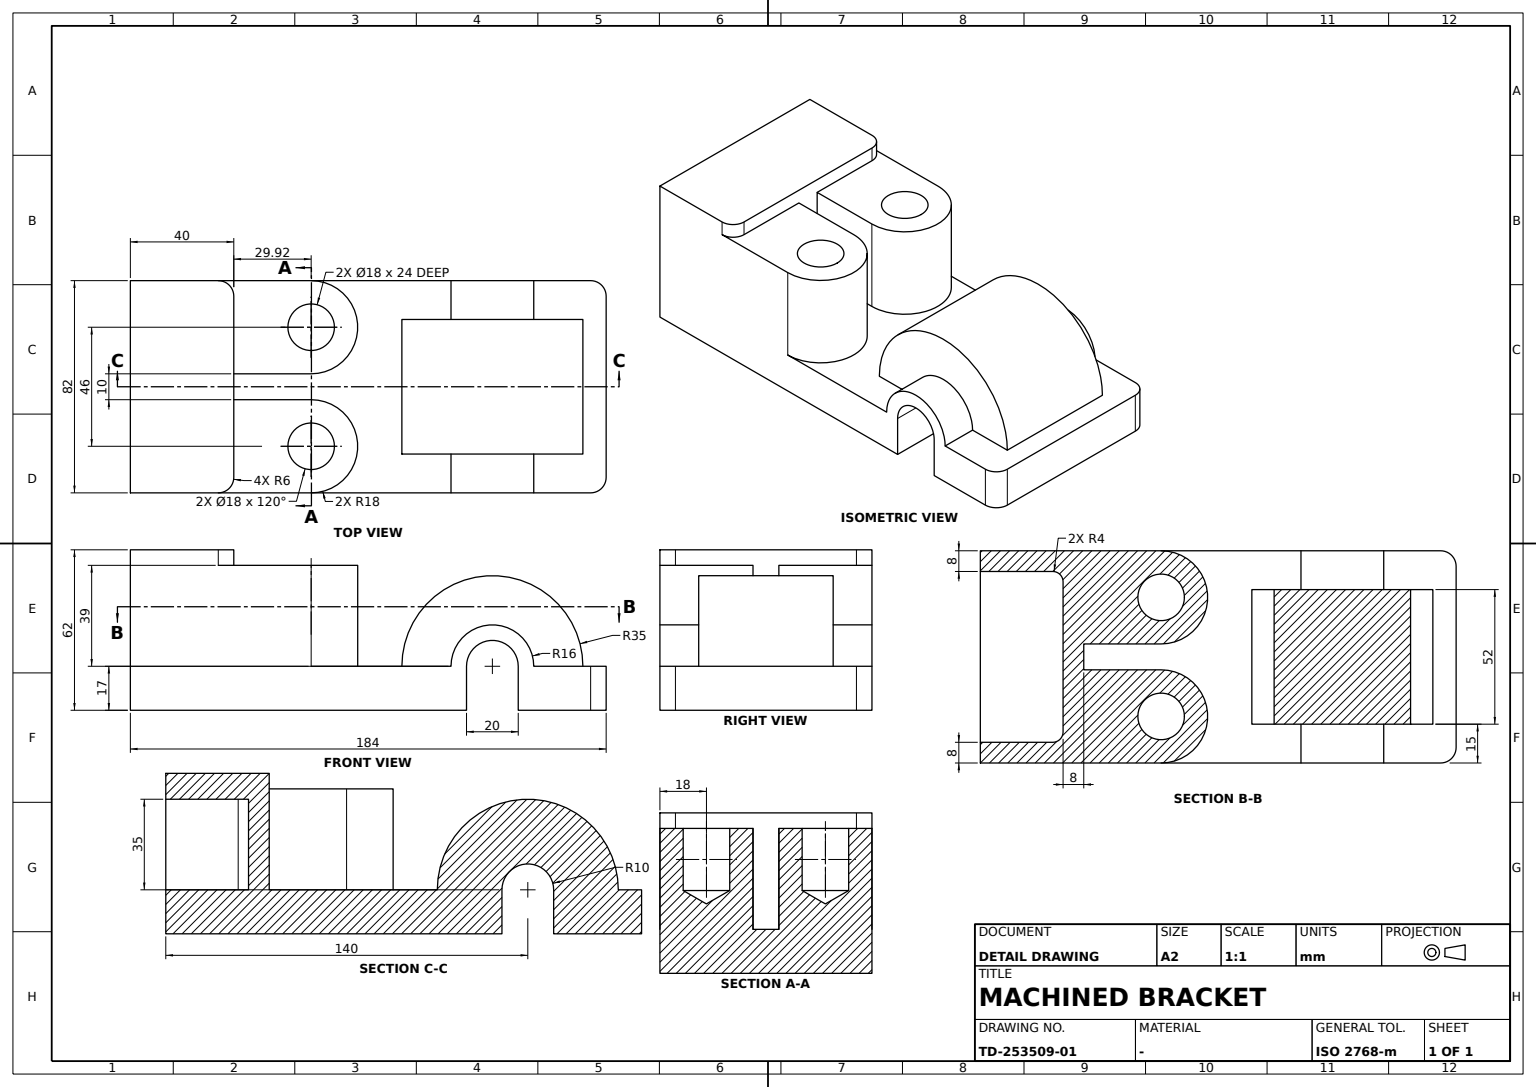
CATIA V5 part; units mm, degrees
sketch "Sketch1" plane through (0, 0, 0) normal (0, 1, 0) x (-1, 0, 0)
  arc A0 (16, 0) -> (-16, 0) centre (0, 0) ccw
  arc A1 (10, 0) -> (-10, 0) centre (0, 0) ccw
  point P0 (0, 10)
  point P1 (-44, 0)
  line L0 (-44, 0) -> (-16, 0)
  line L1 (140, 0) -> (140, -17)
  line L2 (140, -17) -> (10, -17)
  line L3 (-44, -17) -> (-44, 0)
  point P2 (140, 0)
  point P3 (-16, 0)
  line L4 (-10, 0) -> (-10, -17)
  point P4 (-10, 0)
  point P5 (-10, -17)
  line L5 (10, 0) -> (10, -17)
  point P6 (10, 0)
  point P7 (16, 0)
  point P8 (-10, 0)
  point P9 (10, 0)
  point P10 (16, 0)
  line L6 (16, 0) -> (100, 0)
  line L7 (-10, -17) -> (-44, -17)
  point P11 (140, 0)
  line L8 (140, 0) -> (140, 45)
  line L9 (140, 45) -> (100, 45)
  line L10 (100, 45) -> (100, 0)
  dimension "radius A1" = 10
  dimension "radius A0" = 16
  dimension "length L3" = 17
  dimension "distance L3 L1" = 184
  dimension "distance y axis L1" = 140
  dimension "distance L2 L9" = 62
  dimension "length L9" = 40
  constraint coincidence A1 P0
  constraint coincidence P0 y-axis
  constraint coincidence P1 x-axis
  constraint coincidence P3 L0
  constraint coincidence P3 A0
  constraint coincidence P4 L0
  constraint coincidence P4 A1
  constraint coincidence P5 L2
  constraint coincidence P6 L0
  constraint coincidence P6 A1
  constraint coincidence P7 L0
  constraint coincidence P7 A0
  constraint coincidence L0 P8
  constraint coincidence L0 P10
  constraint coincidence L0 L6
  constraint coincidence L2 L7
  constraint coincidence L1 L8
  constraint coincidence P11 P2
  constraint coincidence P4 P8
  constraint coincidence P6 P9
  constraint horizontal L0 x-axis
  constraint horizontal L2 x-axis
  constraint horizontal L6 x-axis
  constraint horizontal L7 x-axis
  constraint horizontal L9 x-axis
  constraint vertical L1 y-axis
  constraint vertical L3 y-axis
  constraint vertical L8 y-axis
  constraint vertical L10 y-axis
  constraint tangency L4 A1
  constraint tangency L5 A1
extrude "Pad1" add sketch "Sketch1" along normal mid plane 82
sketch "Sketch2" plane through (0, 0, 0) normal (0, 1, 0) x (-1, 0, 0)
  arc A0 (35, 0) -> (-35, 0) centre (0, 0) ccw
  arc A1 (16, 0) -> (-16, 0) centre (0, 0) ccw
  point P0 (16, 0)
  point P1 (-16, 0)
  line L0 (-16, 0) -> (-35, 0)
  point P2 (-35, 0)
  point P3 (35, 0)
  point P4 (16, 0)
  line L1 (16, 0) -> (35, 0)
  dimension "radius A0" = 35
  constraint horizontal L0 x-axis
  constraint symmetry P2 P3 y-axis
  constraint symmetry P1 P4 y-axis
  constraint symmetry L0 L1 y-axis
  constraint coincidence P4 P0
extrude "Pad2" add sketch "Sketch2" along normal mid plane 52
sketch "Sketch3" plane through (0, 0, 45) normal (0, 0, 1) x (1, 0, 0)
  line L0 (-140, 33) -> (-112, 33)
  point P0 (-140, 33)
  line L1 (-108, 29) -> (-108, -29)
  line L2 (-112, -33) -> (-140, -33)
  point P1 (-140, -33)
  line L3 (-140, -41) -> (-100, -41) construction
  line L4 (-140, -41) -> (-140, 41) construction
  line L5 (-140, -41) -> (-140, 41) construction
  line L6 (-100, -41) -> (-100, 41) construction
  line L7 (-140, 41) -> (-100, 41) construction
  line L8 (-140, 33) -> (-140, -33)
  arc A0 (-112, 33) -> (-108, 29) centre (-112, 29) cw
  arc A1 (-108, -29) -> (-112, -33) centre (-112, -29) cw
  dimension "distance L2 L3" = 8
  dimension "distance L6 L1" = 8
  dimension "distance L0 L7" = 8
  dimension "radius A0" = 4
  dimension "radius A1" = 4
  constraint horizontal L0 x-axis
  constraint horizontal L2 x-axis
  constraint vertical L1 y-axis
  constraint vertical L8 y-axis
  constraint coincidence L4 P1
  constraint coincidence P0 L5
  constraint tangency A0 L0
  constraint tangency A0 L1
  constraint tangency A1 L1
  constraint tangency A1 L2
extrude "Pocket1" cut sketch "Sketch3" against normal blind 45
fillet "Fillet1" radius 6 4 edges at (-100, 41, 22.5) (-100, -41, 22.5) (44, 41, -8.5) (44, -41, -8.5)
sketch "Sketch4" plane through (0, 0, 0) normal (0, 0, 1) x (1, 0, 0)
  arc A0 (-70.0807, 5) -> (-70.0807, 41) centre (-70.0807, 23) ccw
  point P0 (-70.0807, 23)
  arc A1 (-70.0807, -41) -> (-70.0807, -5) centre (-70.0807, -23) ccw
  point P1 (-70.0807, -23)
  line L0 (-100, -41) -> (-16, -41) construction
  line L1 (-16, 41) -> (-100, 41) construction
  arc A2 (-100, 35) -> (-106, 41) centre (-106, 35) ccw
  point P2 (-100, 35)
  point P3 (-106, 41)
  line L2 (-100, -35) -> (-100, 35) construction
  line L3 (-100, -35) -> (-100, -5)
  line L4 (-100, 5) -> (-100, 35)
  point P4 (-100, -35)
  point P5 (-100, 35)
  arc A3 (-106, -41) -> (-100, -35) centre (-106, -35) ccw
  point P6 (-106, -41)
  point P7 (-100, -35)
  line L5 (-106, -41) -> (-16, -41) construction
  line L6 (-106, -41) -> (-70.0807, -41)
  point P8 (-106, -41)
  line L7 (-16, 41) -> (-106, 41) construction
  line L8 (-70.0807, 41) -> (-106, 41)
  point P9 (-106, 41)
  point P10 (-70.0807, 41)
  point P11 (-70.0807, -41)
  line L9 (-70.0807, -5) -> (-100, -5)
  point P12 (-100, -5)
  line L10 (-70.0807, 5) -> (-100, 5)
  point P13 (-100, 5)
  point P14 (-70.0807, -41)
  point P15 (-70.0807, 41)
  dimension "distance P1 P0" = 46
  dimension "radius A0" = 18
  dimension "radius A1" = 18
  constraint tangency A1 L0
  constraint tangency A0 L1
  constraint tangency L9 A1
  constraint tangency L10 A0
  constraint coincidence A0 P10
  constraint coincidence A1 P11
  constraint coincidence P12 L2
  constraint coincidence P13 L2
  constraint coincidence L5 P14
  constraint coincidence L7 P15
  constraint coincidence P2 P5
  constraint coincidence P3 P9
  constraint coincidence P4 P7
  constraint coincidence P6 P8
  constraint coincidence P10 P15
  constraint coincidence P11 P14
extrude "Pad3" add sketch "Sketch4" along normal blind 39
sketch "Sketch5" plane through (-71.1707, 20.8664, 39) normal (0, 0, 1) x (1, 0, 0)
  point P0 (1.09, 2.1336)
  arc A0 (1.09, -15.8664) -> (1.09, 20.1336) centre (1.09, 2.1336) ccw construction
  constraint concentricity P0 A0
hole "Hole1" at (-70.0807, 23, 39) direction (0, 0, -1) diameter 18 depth 24 tip angle 120
mirror "Mirror1" about plane through (0, 0, 0) normal (0, 1, 0) of "Hole1"
sketch "Sketch6" plane through (0, 0, 45) normal (0, 0, 1) x (1, 0, 0)
  line L0 (-140, 41) -> (-106, 41)
  line L1 (-140, -33) -> (-140, 33)
  point P0 (-140, -33)
  point P1 (-140, 33)
  arc A0 (-100, 35) -> (-106, 41) centre (-106, 35) ccw
  line L2 (-100, -35) -> (-100, 35)
  arc A1 (-106, -41) -> (-100, -35) centre (-106, -35) ccw
  line L3 (-140, -41) -> (-106, -41)
  line L4 (-140, -41) -> (-140, -33)
  point P2 (-140, -33)
  line L5 (-140, 33) -> (-140, 41)
  point P3 (-140, 33)
  constraint vertical L1 y-axis
  constraint coincidence P0 P2
  constraint coincidence P1 P3
extrude "Pad4" add sketch "Sketch6" against normal blind 10
